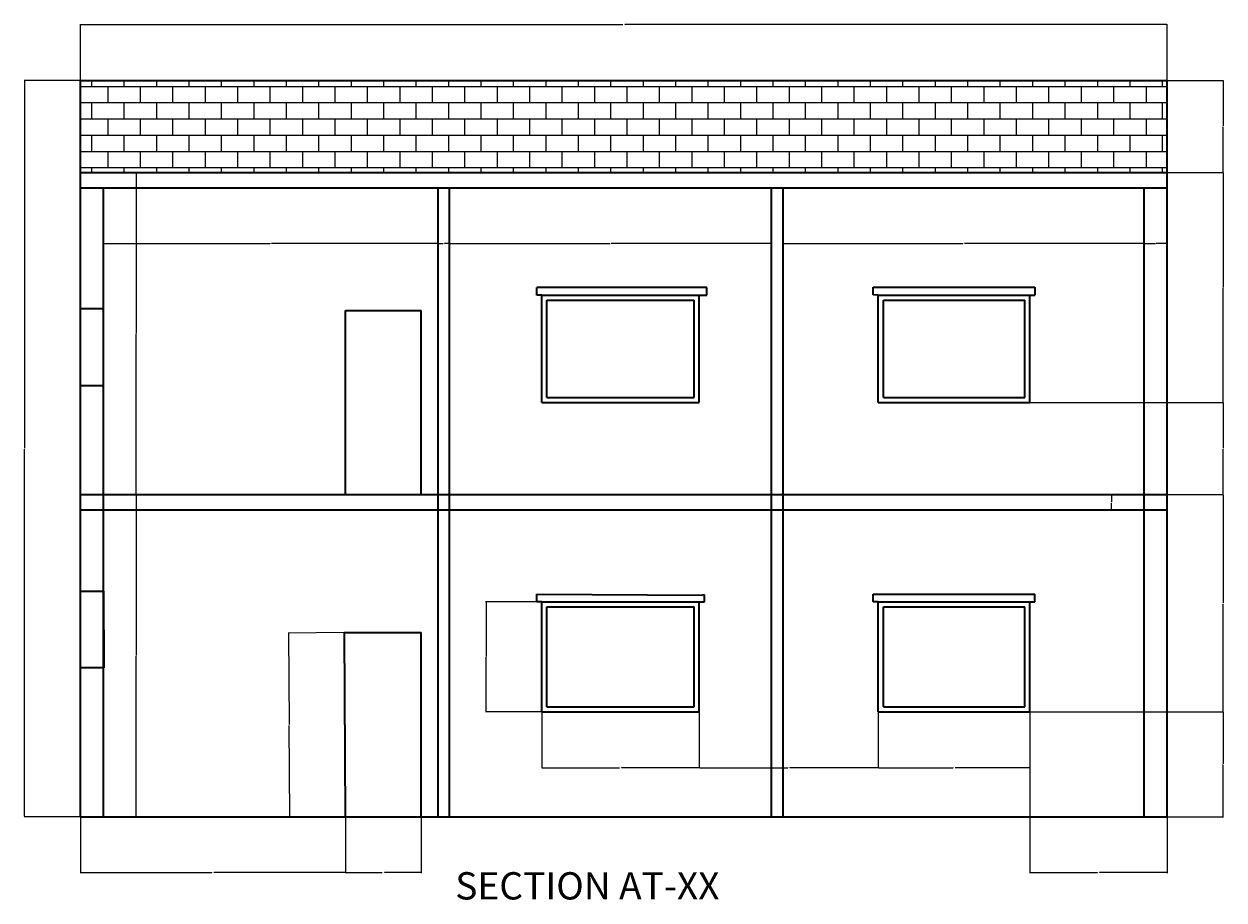
# Model space of a CAD drawing. Units: inches. Extents: x -45 to 1424, y 648 to 1662.
# Tile 4 of 8: x 18 to 488, y 1238 to 1580. Entities that reach past the tile are written whole.
import ezdxf

# ---------------------------------------------------------------- set-up
doc = ezdxf.new("R2010")
doc.units = ezdxf.units.IN
for name, color, linetype, lineweight in [('A-ANNO-DIMS', 2, 'Continuous', 18), ('A-ANNO-TITL', 7, 'Continuous', 35), ('A-SECT', 7, 'Continuous', 35), ('A-WALL-PATT', 6, 'Continuous', 13)]:
    doc.layers.add(name, color=color, linetype=linetype, lineweight=lineweight)
doc.styles.get("Standard").update_dxf_attribs({"font": 'arial.ttf'})
doc.dimstyles.get("Standard").update_dxf_attribs({"dimtxt": 0.18, "dimasz": 0.18, "dimexe": 0.18, "dimexo": 0.0625, "dimgap": 0.09, "dimtad": 0, "dimtih": 1, "dimtoh": 1, "dimdec": 4, "dimzin": 0, "dimdsep": 46, "dimtxsty": 'Standard', "dimcen": 0.09, "dimadec": 0, "dimazin": 0, "dimtfac": 1, "dimtdec": 4, "dimtofl": 0, "dimtmove": 0, "dimatfit": 3, "dimfxl": 1, "dimtolj": 1, "dimtzin": 0, "dimarcsym": 0})

# ---------------------------------------------------------------- blocks, each defined once
blk = doc.blocks.new('*D95')
at = {"layer": 'A-ANNO-DIMS', "color": 0, "lineweight": -2, "transparency": 16777216}
for p, q in [((40, 1558.18), (40, 1580.15)), ((40.18, 1579.97), (252.3, 1579.97)), ((465.22, 1579.97), (253.1, 1579.97)), ((465.4, 1558.18), (465.4, 1580.15))]:
    blk.add_line(p, q, dxfattribs=at)
at = {"layer": 'A-ANNO-DIMS', "color": 0, "transparency": 16777216}
for points in [[(40.18, 1580), (40.18, 1579.94), (40, 1579.97)], [(465.22, 1580), (465.22, 1579.94), (465.4, 1579.97)]]:
    blk.add_solid(points, dxfattribs=at)
at = {"layer": 'Defpoints', "color": 0, "transparency": 16777216}
for p in [(465.4, 1579.97), (40, 1558.12), (465.4, 1558.12)]:
    blk.add_point(p, dxfattribs=at)
at = {"layer": 'A-ANNO-DIMS', "color": 0, "transparency": 16777216, "insert": (252.7, 1579.97), "char_height": 0.18, "attachment_point": 5}
blk.add_mtext('\\A1;425.4', dxfattribs=at)
blk = doc.blocks.new('*D96')
at = {"layer": 'A-ANNO-DIMS', "color": 0, "lineweight": -2, "transparency": 16777216}
for p, q in [((39.94, 1558.12), (17.97, 1558.12)), ((18.15, 1557.94), (18.15, 1414.3)), ((18.15, 1270.3), (18.15, 1413.94)), ((39.94, 1270.12), (17.97, 1270.12))]:
    blk.add_line(p, q, dxfattribs=at)
at = {"layer": 'A-ANNO-DIMS', "color": 0, "transparency": 16777216}
for points in [[(18.12, 1557.94), (18.18, 1557.94), (18.15, 1558.12)], [(18.12, 1270.3), (18.18, 1270.3), (18.15, 1270.12)]]:
    blk.add_solid(points, dxfattribs=at)
at = {"layer": 'Defpoints', "color": 0, "transparency": 16777216}
for p in [(40, 1558.12), (18.15, 1270.12), (40, 1270.12)]:
    blk.add_point(p, dxfattribs=at)
at = {"layer": 'A-ANNO-DIMS', "color": 0, "transparency": 16777216, "insert": (18.15, 1414.12), "char_height": 0.18, "attachment_point": 5}
blk.add_mtext('\\A1;288', dxfattribs=at)
blk = doc.blocks.new('*D97')
at = {"layer": 'A-ANNO-DIMS', "color": 0, "lineweight": -2, "transparency": 16777216}
for p, q in [((411.68, 1311.16), (487.43, 1311.16)), ((487.25, 1310.98), (487.25, 1290.82)), ((487.25, 1270.3), (487.25, 1290.46)), ((465.46, 1270.12), (487.43, 1270.12))]:
    blk.add_line(p, q, dxfattribs=at)
at = {"layer": 'A-ANNO-DIMS', "color": 0, "transparency": 16777216}
for points in [[(487.22, 1310.98), (487.28, 1310.98), (487.25, 1311.16)], [(487.22, 1270.3), (487.28, 1270.3), (487.25, 1270.12)]]:
    blk.add_solid(points, dxfattribs=at)
at = {"layer": 'Defpoints', "color": 0, "transparency": 16777216}
for p in [(411.62, 1311.16), (487.25, 1311.16), (465.4, 1270.12)]:
    blk.add_point(p, dxfattribs=at)
at = {"layer": 'A-ANNO-DIMS', "color": 0, "transparency": 16777216, "insert": (487.25, 1290.64), "char_height": 0.18, "attachment_point": 5}
blk.add_mtext('\\A1;41.04', dxfattribs=at)
blk = doc.blocks.new('*D98')
at = {"layer": 'A-ANNO-DIMS', "color": 0, "lineweight": -2, "transparency": 16777216}
for p, q in [((465.46, 1396.12), (487.43, 1396.12)), ((487.25, 1395.94), (487.25, 1353.82)), ((487.25, 1311.34), (487.25, 1353.46)), ((411.68, 1311.16), (487.43, 1311.16))]:
    blk.add_line(p, q, dxfattribs=at)
at = {"layer": 'A-ANNO-DIMS', "color": 0, "transparency": 16777216}
for points in [[(487.22, 1395.94), (487.28, 1395.94), (487.25, 1396.12)], [(487.22, 1311.34), (487.28, 1311.34), (487.25, 1311.16)]]:
    blk.add_solid(points, dxfattribs=at)
at = {"layer": 'Defpoints', "color": 0, "transparency": 16777216}
for p in [(465.4, 1396.12), (487.25, 1396.12), (411.62, 1311.16)]:
    blk.add_point(p, dxfattribs=at)
at = {"layer": 'A-ANNO-DIMS', "color": 0, "transparency": 16777216, "insert": (487.25, 1353.64), "char_height": 0.18, "attachment_point": 5}
blk.add_mtext('\\A1;84.96', dxfattribs=at)
blk = doc.blocks.new('*D99')
at = {"layer": 'A-ANNO-DIMS', "color": 0, "lineweight": -2, "transparency": 16777216}
for p, q in [((411.68, 1432.12), (487.43, 1432.12)), ((487.25, 1431.94), (487.25, 1414.3)), ((487.25, 1396.3), (487.25, 1413.94)), ((465.46, 1396.12), (487.43, 1396.12))]:
    blk.add_line(p, q, dxfattribs=at)
at = {"layer": 'A-ANNO-DIMS', "color": 0, "transparency": 16777216}
for points in [[(487.22, 1431.94), (487.28, 1431.94), (487.25, 1432.12)], [(487.22, 1396.3), (487.28, 1396.3), (487.25, 1396.12)]]:
    blk.add_solid(points, dxfattribs=at)
at = {"layer": 'Defpoints', "color": 0, "transparency": 16777216}
for p in [(411.62, 1432.12), (487.25, 1432.12), (465.4, 1396.12)]:
    blk.add_point(p, dxfattribs=at)
at = {"layer": 'A-ANNO-DIMS', "color": 0, "transparency": 16777216, "insert": (487.25, 1414.12), "char_height": 0.18, "attachment_point": 5}
blk.add_mtext('\\A1;36', dxfattribs=at)
blk = doc.blocks.new('*D100')
at = {"layer": 'A-ANNO-DIMS', "color": 0, "lineweight": -2, "transparency": 16777216}
for p, q in [((465.46, 1522.12), (487.43, 1522.12)), ((487.25, 1521.94), (487.25, 1477.3)), ((487.25, 1432.3), (487.25, 1476.94)), ((411.68, 1432.12), (487.43, 1432.12))]:
    blk.add_line(p, q, dxfattribs=at)
at = {"layer": 'A-ANNO-DIMS', "color": 0, "transparency": 16777216}
for points in [[(487.22, 1521.94), (487.28, 1521.94), (487.25, 1522.12)], [(487.22, 1432.3), (487.28, 1432.3), (487.25, 1432.12)]]:
    blk.add_solid(points, dxfattribs=at)
at = {"layer": 'Defpoints', "color": 0, "transparency": 16777216}
for p in [(465.4, 1522.12), (487.25, 1522.12), (411.62, 1432.12)]:
    blk.add_point(p, dxfattribs=at)
at = {"layer": 'A-ANNO-DIMS', "color": 0, "transparency": 16777216, "insert": (487.25, 1477.12), "char_height": 0.18, "attachment_point": 5}
blk.add_mtext('\\A1;90', dxfattribs=at)
blk = doc.blocks.new('*D101')
at = {"layer": 'A-ANNO-DIMS', "color": 0, "lineweight": -2, "transparency": 16777216}
for p, q in [((465.46, 1558.12), (487.43, 1558.12)), ((487.25, 1557.94), (487.25, 1540.3)), ((487.25, 1522.3), (487.25, 1539.94)), ((465.46, 1522.12), (487.43, 1522.12))]:
    blk.add_line(p, q, dxfattribs=at)
at = {"layer": 'A-ANNO-DIMS', "color": 0, "transparency": 16777216}
for points in [[(487.22, 1557.94), (487.28, 1557.94), (487.25, 1558.12)], [(487.22, 1522.3), (487.28, 1522.3), (487.25, 1522.12)]]:
    blk.add_solid(points, dxfattribs=at)
at = {"layer": 'Defpoints', "color": 0, "transparency": 16777216}
for p in [(465.4, 1558.12), (487.25, 1558.12), (465.4, 1522.12)]:
    blk.add_point(p, dxfattribs=at)
at = {"layer": 'A-ANNO-DIMS', "color": 0, "transparency": 16777216, "insert": (487.25, 1540.12), "char_height": 0.18, "attachment_point": 5}
blk.add_mtext('\\A1;36', dxfattribs=at)
blk = doc.blocks.new('*D102')
at = {"layer": 'A-ANNO-DIMS', "color": 0, "lineweight": -2, "transparency": 16777216}
for p, q in [((40.06, 1396.12), (62.03, 1396.12)), ((61.85, 1395.94), (61.85, 1333.3)), ((61.85, 1270.3), (61.85, 1332.94)), ((40.06, 1270.12), (62.03, 1270.12))]:
    blk.add_line(p, q, dxfattribs=at)
at = {"layer": 'A-ANNO-DIMS', "color": 0, "transparency": 16777216}
for points in [[(61.82, 1395.94), (61.88, 1395.94), (61.85, 1396.12)], [(61.82, 1270.3), (61.88, 1270.3), (61.85, 1270.12)]]:
    blk.add_solid(points, dxfattribs=at)
at = {"layer": 'Defpoints', "color": 0, "transparency": 16777216}
for p in [(40, 1396.12), (40, 1270.12), (61.85, 1270.12)]:
    blk.add_point(p, dxfattribs=at)
at = {"layer": 'A-ANNO-DIMS', "color": 0, "transparency": 16777216, "insert": (61.85, 1333.12), "char_height": 0.18, "attachment_point": 5}
blk.add_mtext('\\A1;126', dxfattribs=at)
blk = doc.blocks.new('*D103')
at = {"layer": 'A-ANNO-DIMS', "color": 0, "lineweight": -2, "transparency": 16777216}
for p, q in [((40.06, 1522.12), (62.03, 1522.12)), ((61.85, 1521.94), (61.85, 1459.3)), ((61.85, 1396.3), (61.85, 1458.94)), ((40.06, 1396.12), (62.03, 1396.12))]:
    blk.add_line(p, q, dxfattribs=at)
at = {"layer": 'A-ANNO-DIMS', "color": 0, "transparency": 16777216}
for points in [[(61.82, 1521.94), (61.88, 1521.94), (61.85, 1522.12)], [(61.82, 1396.3), (61.88, 1396.3), (61.85, 1396.12)]]:
    blk.add_solid(points, dxfattribs=at)
at = {"layer": 'Defpoints', "color": 0, "transparency": 16777216}
for p in [(40, 1522.12), (40, 1396.12), (61.85, 1396.12)]:
    blk.add_point(p, dxfattribs=at)
at = {"layer": 'A-ANNO-DIMS', "color": 0, "transparency": 16777216, "insert": (61.85, 1459.12), "char_height": 0.18, "attachment_point": 5}
blk.add_mtext('\\A1;126', dxfattribs=at)
blk = doc.blocks.new('*D104')
at = {"layer": 'A-ANNO-DIMS', "color": 0, "lineweight": -2, "transparency": 16777216}
for p, q in [((40, 1270.06), (40, 1248.09)), ((143.79, 1270.06), (143.79, 1248.09)), ((40.18, 1248.27), (91.44, 1248.27)), ((143.61, 1248.27), (92.35, 1248.27))]:
    blk.add_line(p, q, dxfattribs=at)
at = {"layer": 'A-ANNO-DIMS', "color": 0, "transparency": 16777216}
for points in [[(40.18, 1248.3), (40.18, 1248.24), (40, 1248.27)], [(143.61, 1248.3), (143.61, 1248.24), (143.79, 1248.27)]]:
    blk.add_solid(points, dxfattribs=at)
at = {"layer": 'Defpoints', "color": 0, "transparency": 16777216}
for p in [(40, 1270.12), (143.79, 1270.12), (143.79, 1248.27)]:
    blk.add_point(p, dxfattribs=at)
at = {"layer": 'A-ANNO-DIMS', "color": 0, "transparency": 16777216, "insert": (91.89, 1248.27), "char_height": 0.18, "attachment_point": 5}
blk.add_mtext('\\A1;103.79', dxfattribs=at)
blk = doc.blocks.new('*D105')
at = {"layer": 'A-ANNO-DIMS', "color": 0, "lineweight": -2, "transparency": 16777216}
for p, q in [((143.79, 1270.06), (143.79, 1248.09)), ((173.43, 1270.06), (173.43, 1248.09)), ((143.97, 1248.27), (158.14, 1248.27)), ((173.25, 1248.27), (159.07, 1248.27))]:
    blk.add_line(p, q, dxfattribs=at)
at = {"layer": 'A-ANNO-DIMS', "color": 0, "transparency": 16777216}
for points in [[(143.97, 1248.3), (143.97, 1248.24), (143.79, 1248.27)], [(173.25, 1248.3), (173.25, 1248.24), (173.43, 1248.27)]]:
    blk.add_solid(points, dxfattribs=at)
at = {"layer": 'Defpoints', "color": 0, "transparency": 16777216}
for p in [(143.79, 1270.12), (173.43, 1270.12), (173.43, 1248.27)]:
    blk.add_point(p, dxfattribs=at)
at = {"layer": 'A-ANNO-DIMS', "color": 0, "transparency": 16777216, "insert": (158.61, 1248.27), "char_height": 0.18, "attachment_point": 5}
blk.add_mtext('\\A1;29.643', dxfattribs=at)
blk = doc.blocks.new('*D106')
at = {"layer": 'A-ANNO-DIMS', "color": 0, "lineweight": -2, "transparency": 16777216}
for p, q in [((411.62, 1311.1), (411.62, 1248.09)), ((465.4, 1270.06), (465.4, 1248.09)), ((411.8, 1248.27), (438.12, 1248.27)), ((465.22, 1248.27), (438.9, 1248.27))]:
    blk.add_line(p, q, dxfattribs=at)
at = {"layer": 'A-ANNO-DIMS', "color": 0, "transparency": 16777216}
for points in [[(411.8, 1248.3), (411.8, 1248.24), (411.62, 1248.27)], [(465.22, 1248.3), (465.22, 1248.24), (465.4, 1248.27)]]:
    blk.add_solid(points, dxfattribs=at)
at = {"layer": 'Defpoints', "color": 0, "transparency": 16777216}
for p in [(411.62, 1311.16), (465.4, 1270.12), (465.4, 1248.27)]:
    blk.add_point(p, dxfattribs=at)
at = {"layer": 'A-ANNO-DIMS', "color": 0, "transparency": 16777216, "insert": (438.51, 1248.27), "char_height": 0.18, "attachment_point": 5}
blk.add_mtext('\\A1;53.78', dxfattribs=at)
blk = doc.blocks.new('*D107')
at = {"layer": 'A-ANNO-DIMS', "color": 0, "lineweight": -2, "transparency": 16777216}
for p, q in [((220.6, 1311.1), (220.6, 1289.13)), ((282.22, 1311.1), (282.22, 1289.13)), ((220.78, 1289.31), (251.02, 1289.31)), ((282.04, 1289.31), (251.81, 1289.31))]:
    blk.add_line(p, q, dxfattribs=at)
at = {"layer": 'A-ANNO-DIMS', "color": 0, "transparency": 16777216}
for points in [[(220.78, 1289.34), (220.78, 1289.28), (220.6, 1289.31)], [(282.04, 1289.34), (282.04, 1289.28), (282.22, 1289.31)]]:
    blk.add_solid(points, dxfattribs=at)
at = {"layer": 'Defpoints', "color": 0, "transparency": 16777216}
for p in [(220.6, 1311.16), (282.22, 1311.16), (220.6, 1289.31)]:
    blk.add_point(p, dxfattribs=at)
at = {"layer": 'A-ANNO-DIMS', "color": 0, "transparency": 16777216, "insert": (251.41, 1289.31), "char_height": 0.18, "attachment_point": 5}
blk.add_mtext('\\A1;61.62', dxfattribs=at)
blk = doc.blocks.new('*D108')
at = {"layer": 'A-ANNO-DIMS', "color": 0, "lineweight": -2, "transparency": 16777216}
for p, q in [((282.22, 1311.1), (282.22, 1289.13)), ((352.28, 1311.1), (352.28, 1289.13)), ((282.4, 1289.31), (316.86, 1289.31)), ((352.1, 1289.31), (317.64, 1289.31))]:
    blk.add_line(p, q, dxfattribs=at)
at = {"layer": 'A-ANNO-DIMS', "color": 0, "transparency": 16777216}
for points in [[(282.4, 1289.34), (282.4, 1289.28), (282.22, 1289.31)], [(352.1, 1289.34), (352.1, 1289.28), (352.28, 1289.31)]]:
    blk.add_solid(points, dxfattribs=at)
at = {"layer": 'Defpoints', "color": 0, "transparency": 16777216}
for p in [(282.22, 1311.16), (352.28, 1311.16), (282.22, 1289.31)]:
    blk.add_point(p, dxfattribs=at)
at = {"layer": 'A-ANNO-DIMS', "color": 0, "transparency": 16777216, "insert": (317.25, 1289.31), "char_height": 0.18, "attachment_point": 5}
blk.add_mtext('\\A1;70.06', dxfattribs=at)
blk = doc.blocks.new('*D109')
at = {"layer": 'A-ANNO-DIMS', "color": 0, "lineweight": -2, "transparency": 16777216}
for p, q in [((352.28, 1311.1), (352.28, 1289.13)), ((411.62, 1311.1), (411.62, 1289.13)), ((352.46, 1289.31), (381.55, 1289.31)), ((411.44, 1289.31), (382.34, 1289.31))]:
    blk.add_line(p, q, dxfattribs=at)
at = {"layer": 'A-ANNO-DIMS', "color": 0, "transparency": 16777216}
for points in [[(352.46, 1289.34), (352.46, 1289.28), (352.28, 1289.31)], [(411.44, 1289.34), (411.44, 1289.28), (411.62, 1289.31)]]:
    blk.add_solid(points, dxfattribs=at)
at = {"layer": 'Defpoints', "color": 0, "transparency": 16777216}
for p in [(352.28, 1311.16), (411.62, 1311.16), (352.28, 1289.31)]:
    blk.add_point(p, dxfattribs=at)
at = {"layer": 'A-ANNO-DIMS', "color": 0, "transparency": 16777216, "insert": (381.95, 1289.31), "char_height": 0.18, "attachment_point": 5}
blk.add_mtext('\\A1;59.34', dxfattribs=at)
blk = doc.blocks.new('*D110')
at = {"layer": 'A-ANNO-DIMS', "color": 0, "lineweight": -2, "transparency": 16777216}
for p, q in [((143.28, 1342.12), (121.31, 1341.98)), ((121.5, 1341.81), (121.72, 1306.17)), ((121.94, 1270.17), (121.72, 1305.81)), ((143.72, 1270.12), (121.76, 1269.99))]:
    blk.add_line(p, q, dxfattribs=at)
at = {"layer": 'A-ANNO-DIMS', "color": 0, "transparency": 16777216}
for points in [[(121.53, 1341.81), (121.47, 1341.81), (121.49, 1341.99)], [(121.97, 1270.17), (121.91, 1270.17), (121.94, 1269.99)]]:
    blk.add_solid(points, dxfattribs=at)
at = {"layer": 'Defpoints', "color": 0, "transparency": 16777216}
for p in [(121.49, 1341.99), (143.34, 1342.12), (143.79, 1270.12)]:
    blk.add_point(p, dxfattribs=at)
at = {"layer": 'A-ANNO-DIMS', "color": 0, "transparency": 16777216, "insert": (121.72, 1305.99), "char_height": 0.18, "attachment_point": 5}
blk.add_mtext('\\A1;72', dxfattribs=at)
blk = doc.blocks.new('*D111')
at = {"layer": 'A-ANNO-DIMS', "color": 0, "lineweight": -2, "transparency": 16777216}
for p, q in [((220.54, 1354.16), (198.57, 1354.16)), ((198.75, 1353.98), (198.75, 1332.84)), ((198.75, 1311.34), (198.75, 1332.48)), ((220.54, 1311.16), (198.57, 1311.16))]:
    blk.add_line(p, q, dxfattribs=at)
at = {"layer": 'A-ANNO-DIMS', "color": 0, "transparency": 16777216}
for points in [[(198.72, 1353.98), (198.78, 1353.98), (198.75, 1354.16)], [(198.72, 1311.34), (198.78, 1311.34), (198.75, 1311.16)]]:
    blk.add_solid(points, dxfattribs=at)
at = {"layer": 'Defpoints', "color": 0, "transparency": 16777216}
for p in [(198.75, 1354.16), (220.6, 1354.16), (220.6, 1311.16)]:
    blk.add_point(p, dxfattribs=at)
at = {"layer": 'A-ANNO-DIMS', "color": 0, "transparency": 16777216, "insert": (198.75, 1332.66), "char_height": 0.18, "attachment_point": 5}
blk.add_mtext('\\A1;43', dxfattribs=at)
blk = doc.blocks.new('*D112')
at = {"layer": 'A-ANNO-DIMS', "color": 0, "lineweight": -2, "transparency": 16777216}
for p, q in [((465.34, 1396.12), (443.37, 1396.12)), ((443.55, 1395.94), (443.55, 1393.3)), ((443.55, 1390.3), (443.55, 1392.94)), ((465.34, 1390.12), (443.37, 1390.12))]:
    blk.add_line(p, q, dxfattribs=at)
at = {"layer": 'A-ANNO-DIMS', "color": 0, "transparency": 16777216}
for points in [[(443.52, 1395.94), (443.58, 1395.94), (443.55, 1396.12)], [(443.52, 1390.3), (443.58, 1390.3), (443.55, 1390.12)]]:
    blk.add_solid(points, dxfattribs=at)
at = {"layer": 'Defpoints', "color": 0, "transparency": 16777216}
for p in [(443.55, 1396.12), (465.4, 1396.12), (465.4, 1390.12)]:
    blk.add_point(p, dxfattribs=at)
at = {"layer": 'A-ANNO-DIMS', "color": 0, "transparency": 16777216, "insert": (443.55, 1393.12), "char_height": 0.18, "attachment_point": 5}
blk.add_mtext('\\A1;6', dxfattribs=at)
blk = doc.blocks.new('*D113')
at = {"layer": 'A-ANNO-DIMS', "color": 0, "lineweight": -2, "transparency": 16777216}
for p, q in [((49, 1516.06), (49, 1494.09)), ((180, 1516.06), (180, 1494.09)), ((49.18, 1494.27), (114.24, 1494.27)), ((179.82, 1494.27), (114.76, 1494.27))]:
    blk.add_line(p, q, dxfattribs=at)
at = {"layer": 'A-ANNO-DIMS', "color": 0, "transparency": 16777216}
for points in [[(49.18, 1494.3), (49.18, 1494.24), (49, 1494.27)], [(179.82, 1494.3), (179.82, 1494.24), (180, 1494.27)]]:
    blk.add_solid(points, dxfattribs=at)
at = {"layer": 'Defpoints', "color": 0, "transparency": 16777216}
for p in [(49, 1516.12), (180, 1516.12), (49, 1494.27)]:
    blk.add_point(p, dxfattribs=at)
at = {"layer": 'A-ANNO-DIMS', "color": 0, "transparency": 16777216, "insert": (114.5, 1494.27), "char_height": 0.18, "attachment_point": 5}
blk.add_mtext('\\A1;131', dxfattribs=at)
blk = doc.blocks.new('*D114')
at = {"layer": 'A-ANNO-DIMS', "color": 0, "lineweight": -2, "transparency": 16777216}
for p, q in [((180, 1516.06), (180, 1494.09)), ((184.5, 1516.06), (184.5, 1494.09)), ((180.18, 1494.27), (181.99, 1494.27)), ((184.32, 1494.27), (182.51, 1494.27))]:
    blk.add_line(p, q, dxfattribs=at)
at = {"layer": 'A-ANNO-DIMS', "color": 0, "transparency": 16777216}
for points in [[(180.18, 1494.3), (180.18, 1494.24), (180, 1494.27)], [(184.32, 1494.3), (184.32, 1494.24), (184.5, 1494.27)]]:
    blk.add_solid(points, dxfattribs=at)
at = {"layer": 'Defpoints', "color": 0, "transparency": 16777216}
for p in [(180, 1516.12), (184.5, 1516.12), (180, 1494.27)]:
    blk.add_point(p, dxfattribs=at)
at = {"layer": 'A-ANNO-DIMS', "color": 0, "transparency": 16777216, "insert": (182.25, 1494.27), "char_height": 0.18, "attachment_point": 5}
blk.add_mtext('\\A1;4.5', dxfattribs=at)
blk = doc.blocks.new('*D115')
at = {"layer": 'A-ANNO-DIMS', "color": 0, "lineweight": -2, "transparency": 16777216}
for p, q in [((184.5, 1516.06), (184.5, 1494.09)), ((310.5, 1516.06), (310.5, 1494.09)), ((184.68, 1494.27), (247.22, 1494.27)), ((310.32, 1494.27), (247.78, 1494.27))]:
    blk.add_line(p, q, dxfattribs=at)
at = {"layer": 'A-ANNO-DIMS', "color": 0, "transparency": 16777216}
for points in [[(184.68, 1494.3), (184.68, 1494.24), (184.5, 1494.27)], [(310.32, 1494.3), (310.32, 1494.24), (310.5, 1494.27)]]:
    blk.add_solid(points, dxfattribs=at)
at = {"layer": 'Defpoints', "color": 0, "transparency": 16777216}
for p in [(184.5, 1516.12), (310.5, 1516.12), (184.5, 1494.27)]:
    blk.add_point(p, dxfattribs=at)
at = {"layer": 'A-ANNO-DIMS', "color": 0, "transparency": 16777216, "insert": (247.5, 1494.27), "char_height": 0.18, "attachment_point": 5}
blk.add_mtext('\\A1;126', dxfattribs=at)
blk = doc.blocks.new('*D116')
at = {"layer": 'A-ANNO-DIMS', "color": 0, "lineweight": -2, "transparency": 16777216}
for p, q in [((315, 1516.06), (315, 1494.09)), ((456.4, 1516.06), (456.4, 1494.09)), ((315.18, 1494.27), (385.32, 1494.27)), ((456.22, 1494.27), (386.08, 1494.27))]:
    blk.add_line(p, q, dxfattribs=at)
at = {"layer": 'A-ANNO-DIMS', "color": 0, "transparency": 16777216}
for points in [[(315.18, 1494.3), (315.18, 1494.24), (315, 1494.27)], [(456.22, 1494.3), (456.22, 1494.24), (456.4, 1494.27)]]:
    blk.add_solid(points, dxfattribs=at)
at = {"layer": 'Defpoints', "color": 0, "transparency": 16777216}
for p in [(315, 1516.12), (456.4, 1516.12), (315, 1494.27)]:
    blk.add_point(p, dxfattribs=at)
at = {"layer": 'A-ANNO-DIMS', "color": 0, "transparency": 16777216, "insert": (385.7, 1494.27), "char_height": 0.18, "attachment_point": 5}
blk.add_mtext('\\A1;141.4', dxfattribs=at)
blk = doc.blocks.new('*D117')
at = {"layer": 'A-ANNO-DIMS', "color": 0, "lineweight": -2, "transparency": 16777216}
for p, q in [((456.4, 1516.06), (456.4, 1494.09)), ((465.4, 1516.06), (465.4, 1494.09)), ((456.58, 1494.27), (460.75, 1494.27)), ((465.22, 1494.27), (461.05, 1494.27))]:
    blk.add_line(p, q, dxfattribs=at)
at = {"layer": 'A-ANNO-DIMS', "color": 0, "transparency": 16777216}
for points in [[(456.58, 1494.3), (456.58, 1494.24), (456.4, 1494.27)], [(465.22, 1494.3), (465.22, 1494.24), (465.4, 1494.27)]]:
    blk.add_solid(points, dxfattribs=at)
at = {"layer": 'Defpoints', "color": 0, "transparency": 16777216}
for p in [(456.4, 1516.12), (465.4, 1516.12), (456.4, 1494.27)]:
    blk.add_point(p, dxfattribs=at)
at = {"layer": 'A-ANNO-DIMS', "color": 0, "transparency": 16777216, "insert": (460.9, 1494.27), "char_height": 0.18, "attachment_point": 5}
blk.add_mtext('\\A1;9', dxfattribs=at)

msp = doc.modelspace()

# ---------------------------------------------------------------- hatches: boundary and pattern name
at = {"layer": 'A-WALL-PATT'}
h = msp.add_hatch(dxfattribs=at)
h.set_pattern_fill('BRICK', color=256)
h.paths.add_polyline_path([(465.4, 1558.1218), (40, 1558.1218), (40, 1522.1218), (465.4, 1522.1218)])

# ---------------------------------------------------------------- linework, layer by layer
at = {"layer": 'A-SECT'}
for p, q in [((40, 1270.1218), (40, 1558.1218)), ((40, 1558.1218), (465.4, 1558.1218)), ((465.4, 1270.1218), (465.4, 1558.1218)), ((40, 1522.1218), (465.4, 1522.1218)), ((40, 1516.1218), (465.4, 1516.1218)), ((49, 1270.1218), (49, 1516.1218)), ((180, 1270.1218), (180, 1516.1218)), ((184.5, 1270.1218), (184.5, 1516.1218)), ((310.5, 1270.1218), (310.5, 1516.1218)), ((315, 1270.1218), (315, 1516.1218)), ((456.4, 1270.1218), (456.4, 1516.1218)), ((285.2212, 1477.1181), (218.6036, 1477.104)), ((218.6036, 1474.1218), (218.6036, 1477.104)), ((285.2212, 1474.1218), (285.2212, 1477.1181)), ((350.2784, 1474.2067), (350.3376, 1477.2061)), ((350.3376, 1477.2061), (413.618, 1477.2061)), ((413.618, 1477.2061), (413.618, 1474.1218)), ((220.6036, 1474.1218), (218.6036, 1474.1218)), ((220.6036, 1474.1218), (282.2212, 1474.1218)), ((220.6036, 1432.1218), (220.6036, 1474.1218)), ((222.6036, 1434.1218), (222.6036, 1472.1218)), ((222.6036, 1472.1218), (280.2212, 1472.1218)), ((280.2212, 1434.1218), (280.2212, 1472.1218)), ((282.2212, 1432.1218), (282.2212, 1474.1218)), ((282.2212, 1474.1218), (285.2212, 1474.1218)), ((352.2766, 1474.1218), (350.2784, 1474.2067)), ((352.2766, 1432.1218), (352.2766, 1474.1218)), ((352.2766, 1474.1218), (411.618, 1474.1218)), ((354.2766, 1434.1218), (354.2766, 1472.1218)), ((354.2766, 1472.1218), (409.618, 1472.1218)), ((409.618, 1434.1218), (409.618, 1472.1218)), ((411.618, 1432.1218), (411.618, 1474.1218)), ((411.618, 1474.1218), (413.618, 1474.1218)), ((49, 1468.8035), (40, 1468.8035)), ((143.7871, 1396.1218), (143.7871, 1468.1218)), ((143.7871, 1396.1218), (143.7871, 1468.1218)), ((143.7871, 1468.1218), (173.4303, 1468.1218)), ((173.4303, 1396.1218), (173.4303, 1468.1218)), ((40, 1438.8418), (49, 1438.8418)), ((222.6036, 1434.1218), (280.2212, 1434.1218)), ((354.2766, 1434.1218), (409.618, 1434.1218)), ((220.6036, 1432.1218), (282.2212, 1432.1218)), ((352.2766, 1432.1218), (411.618, 1432.1218)), ((40, 1396.1218), (465.4, 1396.1218)), ((40, 1390.1218), (465.4, 1390.1218)), ((40, 1358.3332), (49, 1358.3332)), ((49, 1358.3332), (49.113, 1328.3334)), ((218.6036, 1354.1629), (218.6036, 1357.1643)), ((218.6036, 1357.1643), (218.771, 1357.1582)), ((220.6036, 1354.1629), (218.6036, 1354.1629)), ((218.771, 1357.1582), (283.5492, 1356.8323)), ((220.6036, 1311.1596), (220.6036, 1354.1629)), ((220.6036, 1354.1629), (282.2212, 1354.1629)), ((282.2212, 1311.1596), (282.2212, 1354.1629)), ((282.2212, 1354.1629), (284.2212, 1354.1629)), ((284.2212, 1356.8522), (283.5492, 1356.8323)), ((284.2212, 1354.1629), (284.2212, 1356.8522)), ((350.2766, 1354.1629), (350.3329, 1357.1623)), ((352.2766, 1354.1629), (350.2766, 1354.1629)), ((350.3329, 1357.1623), (413.618, 1357.1623)), ((352.2766, 1311.1596), (352.2766, 1354.1629)), ((352.2766, 1354.1629), (411.618, 1354.1629)), ((411.618, 1311.1596), (411.618, 1354.1629)), ((411.618, 1354.1629), (413.618, 1354.1629)), ((413.618, 1354.1629), (413.618, 1357.1623)), ((222.6036, 1352.1629), (280.2212, 1352.1629)), ((222.6036, 1313.1596), (222.6036, 1352.1629)), ((280.2212, 1313.1596), (280.2212, 1352.1629)), ((354.2766, 1352.1629), (409.618, 1352.1629)), ((354.2766, 1313.1596), (354.2766, 1352.1629)), ((409.618, 1313.1596), (409.618, 1352.1629)), ((143.7871, 1270.1218), (143.3444, 1342.1204)), ((143.3444, 1342.1204), (173.4303, 1342.1204)), ((173.4303, 1270.1218), (173.4303, 1342.1204)), ((49.113, 1328.3334), (40, 1328.3334)), ((220.6036, 1311.1596), (282.2212, 1311.1596)), ((222.6036, 1313.1596), (280.2212, 1313.1596)), ((352.2766, 1311.1596), (411.618, 1311.1596)), ((354.2766, 1313.1596), (409.618, 1313.1596)), ((40, 1270.1218), (465.4, 1270.1218))]:
    msp.add_line(p, q, dxfattribs=at)

# ---------------------------------------------------------------- texts
at = {"layer": 'A-ANNO-TITL', "insert": (186.6961, 1248.4393), "char_height": 10.673289, "attachment_point": 1}
msp.add_mtext('SECTION AT-XX', dxfattribs=at)

# ---------------------------------------------------------------- dimensions: what is measured, and where the dimension line sits
at = {"layer": 'A-ANNO-DIMS'}
for base, p1, p2, override, picture, middle in [((465.4, 1579.9718), (40, 1558.1218), (465.4, 1558.1218), {"dimdec": 1, "dimlfac": 1, "dimrnd": 0, "dimzin": 0, "dimdsep": 46, "dimlunit": 2}, '*D95', (252.7, 1579.9718)), ((465.4, 1248.2718), (411.618, 1311.1596), (465.4, 1270.1218), {"dimdec": 2, "dimlfac": 1, "dimrnd": 0, "dimzin": 0, "dimdsep": 46, "dimlunit": 2}, '*D106', (438.509, 1248.2718)), ((143.7871, 1248.2718), (40, 1270.1218), (143.7871, 1270.1218), {"dimdec": 2, "dimlfac": 1, "dimrnd": 0, "dimzin": 0, "dimdsep": 46, "dimlunit": 2}, '*D104', (91.8936, 1248.2718)), ((173.4303, 1248.2718), (143.7871, 1270.1218), (173.4303, 1270.1218), {"dimdec": 3, "dimlfac": 1, "dimrnd": 0, "dimzin": 0, "dimdsep": 46, "dimlunit": 2}, '*D105', (158.6087, 1248.2718))]:
    dim = msp.add_linear_dim(base=base, p1=p1, p2=p2, dimstyle='Standard', override=override, dxfattribs=at)
    dim.commit()
    dim.dimension.update_dxf_attribs({"geometry": picture, "text_midpoint": middle})
for base, p1, p2, angle, override, picture, middle in [((18.15, 1270.1218), (40, 1558.1218), (40, 1270.1218), 90, {"dimdec": 0, "dimlfac": 1, "dimrnd": 0, "dimzin": 0, "dimdsep": 46, "dimlunit": 2}, '*D96', (18.15, 1414.1218)), ((487.25, 1558.1218), (465.4, 1522.1218), (465.4, 1558.1218), 90, {"dimdec": 0, "dimlfac": 1, "dimrnd": 0, "dimzin": 0, "dimdsep": 46, "dimlunit": 2}, '*D101', (487.25, 1540.1218)), ((61.85, 1396.1218), (40, 1522.1218), (40, 1396.1218), 270, {"dimdec": 0, "dimlfac": 1, "dimrnd": 0, "dimzin": 0, "dimdsep": 46, "dimlunit": 2}, '*D103', (61.85, 1459.1218)), ((487.25, 1522.1218), (411.618, 1432.1218), (465.4, 1522.1218), 90, {"dimdec": 0, "dimlfac": 1, "dimrnd": 0, "dimzin": 0, "dimdsep": 46, "dimlunit": 2}, '*D100', (487.25, 1477.1218)), ((49, 1494.2718), (180, 1516.1218), (49, 1516.1218), 180, {"dimdec": 0, "dimlfac": 1, "dimrnd": 0, "dimzin": 0, "dimdsep": 46, "dimlunit": 2}, '*D113', (114.5, 1494.2718)), ((180, 1494.2718), (184.5, 1516.1218), (180, 1516.1218), 180, {"dimdec": 1, "dimlfac": 1, "dimrnd": 0, "dimzin": 0, "dimdsep": 46, "dimlunit": 2}, '*D114', (182.25, 1494.2718)), ((184.5, 1494.2718), (310.5, 1516.1218), (184.5, 1516.1218), 180, {"dimdec": 0, "dimlfac": 1, "dimrnd": 0, "dimzin": 0, "dimdsep": 46, "dimlunit": 2}, '*D115', (247.5, 1494.2718)), ((315, 1494.2718), (456.4, 1516.1218), (315, 1516.1218), 180, {"dimdec": 1, "dimlfac": 1, "dimrnd": 0, "dimzin": 0, "dimdsep": 46, "dimlunit": 2}, '*D116', (385.7, 1494.2718)), ((456.4, 1494.2718), (465.4, 1516.1218), (456.4, 1516.1218), 180, {"dimdec": 0, "dimlfac": 1, "dimrnd": 0, "dimzin": 0, "dimdsep": 46, "dimlunit": 2}, '*D117', (460.9, 1494.2718)), ((487.25, 1432.1218), (465.4, 1396.1218), (411.618, 1432.1218), 90, {"dimdec": 0, "dimlfac": 1, "dimrnd": 0, "dimzin": 0, "dimdsep": 46, "dimlunit": 2}, '*D99', (487.25, 1414.1218)), ((61.85, 1270.1218), (40, 1396.1218), (40, 1270.1218), 270, {"dimdec": 0, "dimlfac": 1, "dimrnd": 0, "dimzin": 0, "dimdsep": 46, "dimlunit": 2}, '*D102', (61.85, 1333.1218)), ((487.25, 1396.1218), (411.618, 1311.1596), (465.4, 1396.1218), 90, {"dimdec": 2, "dimlfac": 1, "dimrnd": 0, "dimzin": 0, "dimdsep": 46, "dimlunit": 2}, '*D98', (487.25, 1353.6407)), ((443.55, 1396.1218), (465.4, 1390.1218), (465.4, 1396.1218), 90, {"dimdec": 0, "dimlfac": 1, "dimrnd": 0, "dimzin": 0, "dimdsep": 46, "dimlunit": 2}, '*D112', (443.55, 1393.1218)), ((198.7536, 1354.1629), (220.6036, 1311.1596), (220.6036, 1354.1629), 90, {"dimdec": 0, "dimlfac": 1, "dimrnd": 0, "dimzin": 0, "dimdsep": 46, "dimlunit": 2}, '*D111', (198.7536, 1332.6612)), ((121.4948, 1341.9861), (143.7871, 1270.1218), (143.3444, 1342.1204), 90.352296, {"dimdec": 0, "dimlfac": 1, "dimrnd": 0, "dimzin": 0, "dimdsep": 46, "dimlunit": 2}, '*D110', (121.7162, 1305.9868)), ((220.6036, 1289.3096), (282.2212, 1311.1596), (220.6036, 1311.1596), 180, {"dimdec": 2, "dimlfac": 1, "dimrnd": 0, "dimzin": 0, "dimdsep": 46, "dimlunit": 2}, '*D107', (251.4124, 1289.3096)), ((282.2212, 1289.3096), (352.2766, 1311.1596), (282.2212, 1311.1596), 180, {"dimdec": 2, "dimlfac": 1, "dimrnd": 0, "dimzin": 0, "dimdsep": 46, "dimlunit": 2}, '*D108', (317.2489, 1289.3096)), ((352.2766, 1289.3096), (411.618, 1311.1596), (352.2766, 1311.1596), 180, {"dimdec": 2, "dimlfac": 1, "dimrnd": 0, "dimzin": 0, "dimdsep": 46, "dimlunit": 2}, '*D109', (381.9473, 1289.3096)), ((487.25, 1311.1596), (465.4, 1270.1218), (411.618, 1311.1596), 90, {"dimdec": 2, "dimlfac": 1, "dimrnd": 0, "dimzin": 0, "dimdsep": 46, "dimlunit": 2}, '*D97', (487.25, 1290.6407))]:
    dim = msp.add_linear_dim(base=base, p1=p1, p2=p2, angle=angle, dimstyle='Standard', override=override, dxfattribs=at)
    dim.commit()
    dim.dimension.update_dxf_attribs({"geometry": picture, "text_midpoint": middle})

doc.saveas('drawing.dxf')
